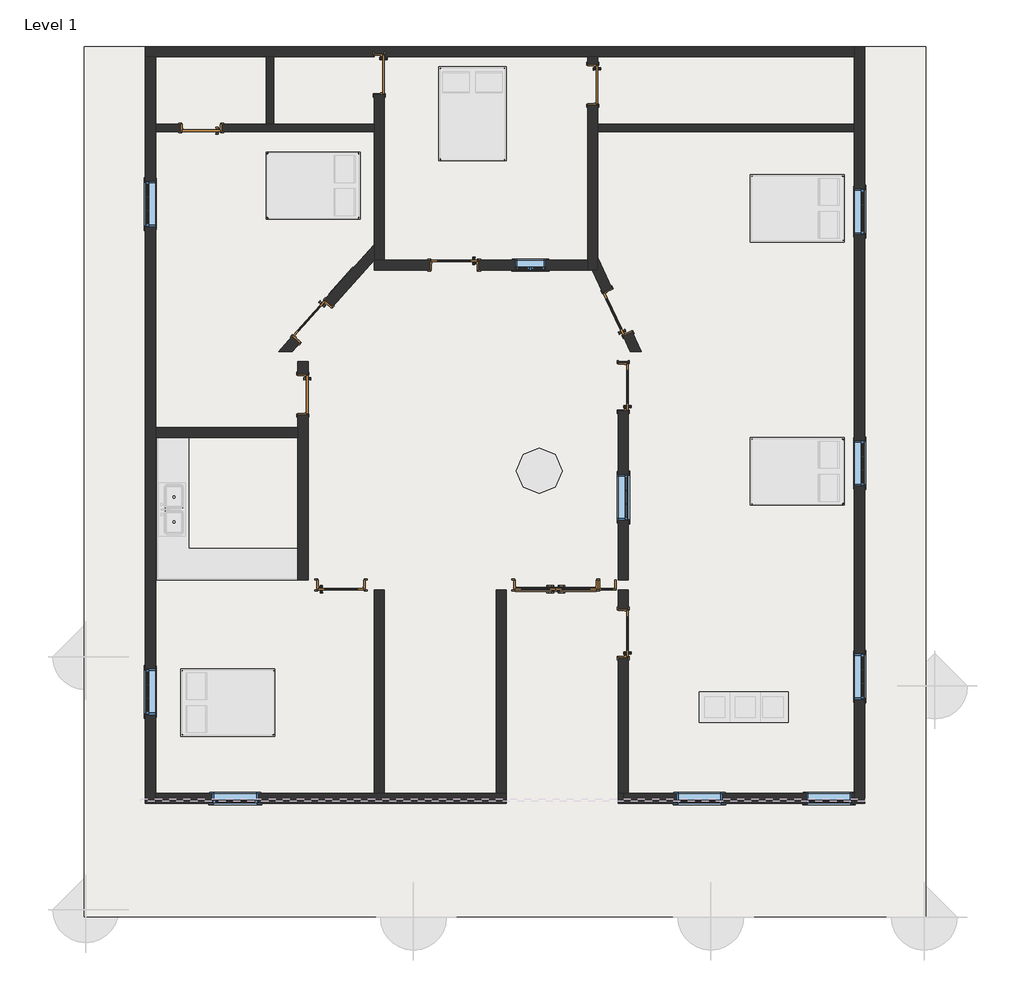
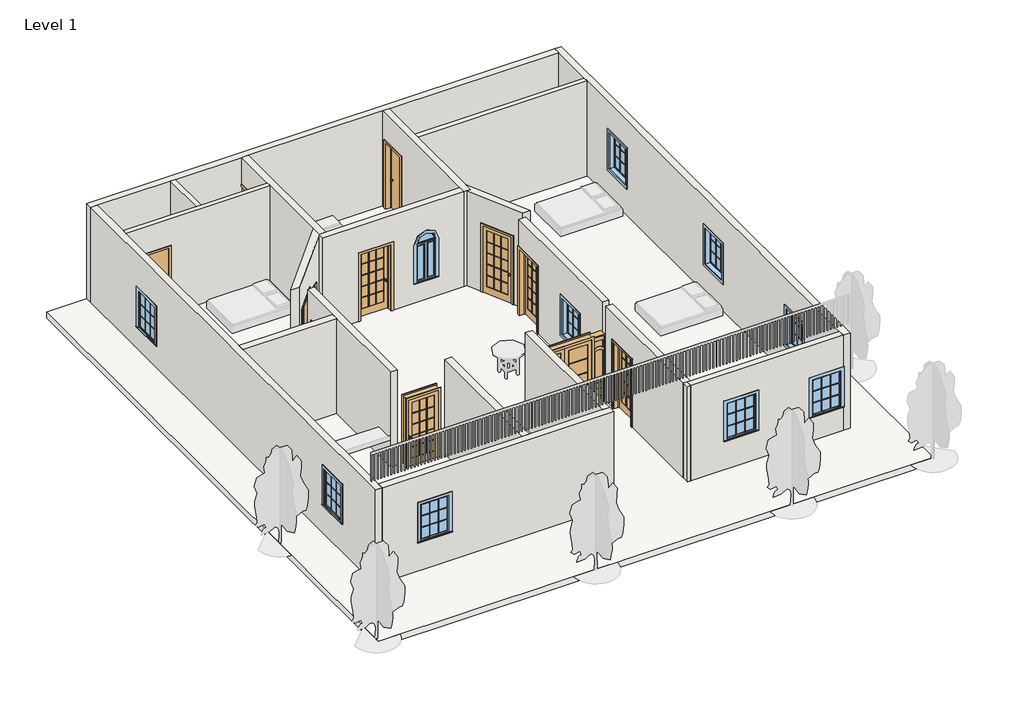
# One storey, part 1 of 3: 19 walls, 12 doors, 11 windows, 1 slab.
"""IFC4 building model written with IfcOpenShell, lengths in millimetres."""

from ifc_helpers import new_model, si_unit, frame, origin, origin_with_axes, place, context, project, spatial, polyline, circle_curve, outline, extrude, faceted_brep, transform, mapped, element, save
from ifc_brep_helpers import plane_surface, revolved_surface, advanced_brep
from components import door_c3736dc5, door_d93d7eea, door_715cd483, door_160b0797, door_6e1855c2, door_cfd81529, window_08a4fb52, window_29c06734, e_49ac7ee0

model = new_model("IFC4")

# Units and contexts
model_context = context("Model", 3, world=origin())
ifc_project = project(units=[si_unit("LENGTHUNIT", "METRE", prefix="MILLI")], contexts=[model_context])

# Site, building, storey
site = spatial("IfcSite", under=ifc_project)
building = spatial("IfcBuilding", under=site)
storey = spatial("IfcBuildingStorey", under=building, Name="Level 1", Elevation=0.0)

# Doors
placement = place(None, origin())
door_shape = door_c3736dc5(model_context)
element("IfcDoor", 1, ObjectType="12\" x 84\"", at=placement, inside=storey, context=model_context, shape_type="MappedRepresentation", body=[
    mapped(door_shape, transform((-305.2097877, 7760.2557946, 0.0), x_axis=(-1.0, 0.0, 0.0), y_axis=(0.0, -1.0, 0.0), z_axis=(0.0, 0.0, 1.0))),
])
door_2_shape = door_d93d7eea(model_context)
element("IfcDoor", 2, ObjectType="Door-Exterior-Double-Full Glass-Wood_Clad : 64\" x 84\"", at=placement, inside=storey, context=model_context, shape_type="MappedRepresentation", body=[
    mapped(door_2_shape, transform((-1333.9097877, 7760.2557946, 0.0), x_axis=(1.0, 0.0, 0.0), y_axis=(0.0, 1.0, 0.0), z_axis=(0.0, 0.0, 1.0))),
])
door_3_shape = door_715cd483(model_context)
element("IfcDoor", 3, ObjectType="Door-Interior-Single-Flush_Panel-Wood : 30\" x 84\"", at=placement, inside=storey, context=model_context, shape_type="MappedRepresentation", body=[
    mapped(door_3_shape, transform((-594.1347877, 17771.0307946, 0.0), x_axis=(0.0, -1.0, 0.0), y_axis=(1.0, 0.0, 0.0), z_axis=(0.0, 0.0, 1.0))),
])
element("IfcDoor", 4, ObjectType="Door-Interior-Single-Flush_Panel-Wood : 30\" x 84\"", at=placement, inside=storey, context=model_context, shape_type="MappedRepresentation", body=[
    mapped(door_3_shape, transform((-6385.3347877, 11573.4307946, 0.0), x_axis=(0.0, -1.0, 0.0), y_axis=(1.0, 0.0, 0.0), z_axis=(0.0, 0.0, 1.0))),
])
element("IfcDoor", 5, ObjectType="Door-Interior-Single-Flush_Panel-Wood : 30\" x 84\"", at=placement, inside=storey, context=model_context, shape_type="MappedRepresentation", body=[
    mapped(door_3_shape, transform((-4861.3347877, 17974.2307946, 0.0), x_axis=(0.0, -1.0, 0.0), y_axis=(1.0, 0.0, 0.0), z_axis=(0.0, 0.0, 1.0))),
])
door_4_shape = door_160b0797(model_context)
element("IfcDoor", 6, ObjectType="Door-Interior-Single-Flush_Panel-Wood : 30\" x 84\"", at=placement, inside=storey, context=model_context, shape_type="MappedRepresentation", body=[
    mapped(door_4_shape, transform((-8420.5097877, 16904.2557946, 0.0), x_axis=(-1.0, 0.0, 0.0), y_axis=(0.0, -1.0, 0.0), z_axis=(0.0, 0.0, 1.0))),
])
door_5_shape = door_6e1855c2(model_context)
element("IfcDoor", 7, ObjectType="Door-Interior-Single-Full Glass-Wood : 36\" x 84\"", at=placement, inside=storey, context=model_context, shape_type="MappedRepresentation", body=[
    mapped(door_5_shape, transform((-5626.5097877, 7760.2557946, 0.0), x_axis=(1.0, 0.0, 0.0), y_axis=(0.0, 1.0, 0.0), z_axis=(0.0, 0.0, 1.0))),
])
element("IfcDoor", 8, ObjectType="Door-Interior-Single-Full Glass-Wood : 36\" x 84\"", at=placement, inside=storey, context=model_context, shape_type="MappedRepresentation", body=[
    mapped(door_5_shape, transform((15.4652123, 11725.8307946, 0.0), x_axis=(0.0, 1.0, 0.0), y_axis=(-1.0, 0.0, 0.0), z_axis=(0.0, 0.0, 1.0))),
])
element("IfcDoor", 9, ObjectType="Door-Interior-Single-Full Glass-Wood : 36\" x 84\"", at=placement, inside=storey, context=model_context, shape_type="MappedRepresentation", body=[
    mapped(door_5_shape, transform((15.4652123, 6798.2307946, 0.0), x_axis=(0.0, 1.0, 0.0), y_axis=(-1.0, 0.0, 0.0), z_axis=(0.0, 0.0, 1.0))),
])
element("IfcDoor", 10, ObjectType="Door-Interior-Single-Full Glass-Wood : 36\" x 84\"", at=placement, inside=storey, context=model_context, shape_type="MappedRepresentation", body=[
    mapped(door_5_shape, transform((-3365.9097877, 14167.4057946, 0.0), x_axis=(-1.0, 0.0, 0.0), y_axis=(0.0, -1.0, 0.0), z_axis=(0.0, 0.0, 1.0))),
])
element("IfcDoor", 11, ObjectType="Door-Interior-Single-Full Glass-Wood : 36\" x 84\"", at=placement, inside=storey, context=model_context, shape_type="MappedRepresentation", body=[
    mapped(door_5_shape, transform((-6206.5889969, 13036.54514, 0.0), x_axis=(-0.666794859469825, -0.7452413135251, 0.0), y_axis=(0.7452413135251, -0.666794859469825, 0.0), z_axis=(0.0, 0.0, 1.0))),
])
door_6_shape = door_cfd81529(model_context)
element("IfcDoor", 12, ObjectType="Door-Interior-Single-Full Glass-Wood : 36\" x 84\"", at=placement, inside=storey, context=model_context, shape_type="MappedRepresentation", body=[
    mapped(door_6_shape, transform((-102.8737328, 13220.5207409, 0.0), x_axis=(-0.4226182617406977, 0.9063077870366507, 0.0), y_axis=(-0.9063077870366507, -0.4226182617406977, 0.0), z_axis=(0.0, 0.0, 1.0))),
])

# Slab
element("IfcSlab", 13, ObjectType="LW Concrete on Metal Deck", at=placement, inside=storey, context=model_context, shape_type="SweptSolid", body=[
    extrude(outline(polyline([(6057.4902123, 18533.0307946), (6057.4902123, 1134.0307946), (-10757.3097877, 1134.0307946), (-10757.3097877, 18533.0307946), (6057.4902123, 18533.0307946)])), frame((0.0, 0.0, -186.0351562), z_axis=(0.0, 0.0, 1.0), x_axis=(1.0, 0.0, 0.0)), (0.0, 0.0, 1.0), 186.0351562),
])

# Walls
element("IfcWall", 14, ObjectType="Generic - 6\"", at=placement, inside=storey, context=model_context, shape_type="Brep", body=[
    faceted_brep([(-9334.9097877, 16831.2307946, 3048.0), (-9334.9097877, 16831.2307946, 0.0), (-8826.9097877, 16831.2307946, 0.0), (-8826.9097877, 16831.2307946, 2159.0), (-8014.1097877, 16831.2307946, 2159.0), (-8014.1097877, 16831.2307946, 0.0), (-4966.1097877, 16831.2307946, 0.0), (-4966.1097877, 16831.2307946, 3048.0), (-9334.9097877, 16983.6307946, 0.0), (-9334.9097877, 16983.6307946, 3048.0), (-7125.1097877, 16983.6307946, 3048.0), (-6972.7097877, 16983.6307946, 3048.0), (-4966.1097877, 16983.6307946, 3048.0), (-4966.1097877, 16983.6307946, 0.0), (-6972.7097877, 16983.6307946, 0.0), (-7125.1097877, 16983.6307946, 0.0), (-8014.1097877, 16983.6307946, 0.0), (-8014.1097877, 16983.6307946, 2159.0), (-8826.9097877, 16983.6307946, 2159.0), (-8826.9097877, 16983.6307946, 0.0)], [[[0, 1, 2, 3, 4, 5, 6, 7]], [[8, 9, 10, 11, 12, 13, 14, 15, 16, 17, 18, 19]], [[1, 8, 19, 2]], [[13, 6, 5, 16, 15, 14]], [[1, 0, 9, 8]], [[7, 6, 13, 12]], [[18, 3, 2, 19]], [[3, 18, 17, 4]], [[4, 17, 16, 5]], [[0, 7, 12, 11, 10, 9]]]),
])
element("IfcWall", 15, ObjectType="Generic - 6\"", at=placement, inside=storey, context=model_context, shape_type="SweptSolid", body=[
    extrude(outline(polyline([(-7125.1097877, 16983.6307946), (-7125.1097877, 18329.8307946), (-6972.7097877, 18329.8307946), (-6972.7097877, 16983.6307946), (-7125.1097877, 16983.6307946)])), origin_with_axes(), (0.0, 0.0, 1.0), 3048.0),
])
element("IfcWall", 16, ObjectType="Generic - 6\"", at=placement, inside=storey, context=model_context, shape_type="SweptSolid", body=[
    extrude(outline(polyline([(4635.0902123, 16831.2307946), (-495.7097877, 16831.2307946), (-495.7097877, 16983.6307946), (4635.0902123, 16983.6307946), (4635.0902123, 16831.2307946)])), origin_with_axes(), (0.0, 0.0, 1.0), 3048.0),
])
element("IfcWall", 17, ObjectType="Generic - 8\"", at=placement, inside=storey, context=model_context, shape_type="Brep", body=[
    faceted_brep([(-9538.1097877, 18329.8307946, 3048.0), (-9538.1097877, 18329.8307946, 0.0), (-9334.9097877, 18329.8307946, 0.0), (-7125.1097877, 18329.8307946, 0.0), (-6972.7097877, 18329.8307946, 0.0), (-4966.1097877, 18329.8307946, 0.0), (-4966.1097877, 18329.8307946, 2159.0), (-4762.9097877, 18329.8307946, 2159.0), (-4762.9097877, 18329.8307946, 0.0), (-698.9097877, 18329.8307946, 0.0), (-495.7097877, 18329.8307946, 0.0), (4635.0902123, 18329.8307946, 0.0), (4635.0902123, 18329.8307946, 3048.0), (-495.7097877, 18329.8307946, 3048.0), (-698.9097877, 18329.8307946, 3048.0), (-4762.9097877, 18329.8307946, 3048.0), (-4966.1097877, 18329.8307946, 3048.0), (-6972.7097877, 18329.8307946, 3048.0), (-7125.1097877, 18329.8307946, 3048.0), (-9334.9097877, 18329.8307946, 3048.0), (4635.0902123, 18533.0307946, 0.0), (-9538.1097877, 18533.0307946, 0.0), (-9538.1097877, 18533.0307946, 3048.0), (4635.0902123, 18533.0307946, 3048.0), (-4762.9097877, 18380.6307946, 0.0), (-4966.1097877, 18380.6307946, 0.0), (-4966.1097877, 18380.6307946, 2159.0), (-4762.9097877, 18380.6307946, 2159.0)], [[[0, 1, 2, 3, 4, 5, 6, 7, 8, 9, 10, 11, 12, 13, 14, 15, 16, 17, 18, 19]], [[20, 21, 22, 23]], [[21, 20, 11, 10, 9, 8, 24, 25, 5, 4, 3, 2, 1]], [[1, 0, 22, 21]], [[12, 11, 20, 23]], [[25, 26, 6, 5]], [[27, 24, 8, 7]], [[26, 27, 7, 6]], [[26, 25, 24, 27]], [[0, 19, 18, 17, 16, 15, 14, 13, 12, 23, 22]]]),
])
element("IfcWall", 18, ObjectType="Generic - 8\"", at=placement, inside=storey, context=model_context, shape_type="Brep", body=[
    faceted_brep([(-9334.9097877, 3394.6307946, 0.0), (-9334.9097877, 3597.8307946, 0.0), (-9334.9097877, 7661.8307946, 0.0), (-9334.9097877, 7865.0307946, 0.0), (-9334.9097877, 10709.8307946, 0.0), (-9334.9097877, 10913.0307946, 0.0), (-9334.9097877, 12233.8307946, 0.0), (-9334.9097877, 12437.0307946, 0.0), (-9334.9097877, 16831.2307946, 0.0), (-9334.9097877, 16983.6307946, 0.0), (-9334.9097877, 18329.8307946, 0.0), (-9334.9097877, 18329.8307946, 3048.0), (-9334.9097877, 16983.6307946, 3048.0), (-9334.9097877, 16831.2307946, 3048.0), (-9334.9097877, 12437.0307946, 3048.0), (-9334.9097877, 12233.8307946, 3048.0), (-9334.9097877, 10913.0307946, 3048.0), (-9334.9097877, 10709.8307946, 3048.0), (-9334.9097877, 7865.0307946, 3048.0), (-9334.9097877, 7661.8307946, 3048.0), (-9334.9097877, 3597.8307946, 3048.0), (-9334.9097877, 3394.6307946, 3048.0), (-9334.9097877, 15840.6307946, 1923.320936), (-9334.9097877, 15840.6307946, 704.120936), (-9334.9097877, 14926.2307946, 704.120936), (-9334.9097877, 14926.2307946, 1923.320936), (-9334.9097877, 6087.0307946, 2133.6), (-9334.9097877, 6087.0307946, 914.4), (-9334.9097877, 5172.6307946, 914.4), (-9334.9097877, 5172.6307946, 2133.6), (-9538.1097877, 3394.6307946, 0.0), (-9538.1097877, 3394.6307946, 3048.0), (-9538.1097877, 18329.8307946, 3048.0), (-9538.1097877, 18329.8307946, 0.0), (-9538.1097877, 15840.6307946, 1923.320936), (-9538.1097877, 14926.2307946, 1923.320936), (-9538.1097877, 14926.2307946, 704.120936), (-9538.1097877, 15840.6307946, 704.120936), (-9538.1097877, 6087.0307946, 2133.6), (-9538.1097877, 5172.6307946, 2133.6), (-9538.1097877, 5172.6307946, 914.4), (-9538.1097877, 6087.0307946, 914.4)], [[[0, 1, 2, 3, 4, 5, 6, 7, 8, 9, 10, 11, 12, 13, 14, 15, 16, 17, 18, 19, 20, 21], [22, 23, 24, 25], [26, 27, 28, 29]], [[30, 31, 32, 33], [34, 35, 36, 37], [38, 39, 40, 41]], [[10, 9, 8, 7, 6, 5, 4, 3, 2, 1, 0, 30, 33]], [[11, 10, 33, 32]], [[0, 21, 31, 30]], [[23, 22, 34, 37]], [[24, 23, 37, 36]], [[25, 24, 36, 35]], [[22, 25, 35, 34]], [[27, 26, 38, 41]], [[28, 27, 41, 40]], [[29, 28, 40, 39]], [[26, 29, 39, 38]], [[21, 20, 19, 18, 17, 16, 15, 14, 13, 12, 11, 32, 31]]]),
])
element("IfcWall", 19, ObjectType="Generic - 8\"", at=placement, inside=storey, context=model_context, shape_type="Brep", body=[
    faceted_brep([(4635.0902123, 18533.0307946, 0.0), (4635.0902123, 18329.8307946, 0.0), (4635.0902123, 16983.6307946, 0.0), (4635.0902123, 16831.2307946, 0.0), (4635.0902123, 12437.0307946, 0.0), (4635.0902123, 12233.8307946, 0.0), (4635.0902123, 7865.0307946, 0.0), (4635.0902123, 7661.8307946, 0.0), (4635.0902123, 3597.8307946, 0.0), (4635.0902123, 3394.6307946, 0.0), (4635.0902123, 3394.6307946, 3048.0), (4635.0902123, 3597.8307946, 3048.0), (4635.0902123, 7661.8307946, 3048.0), (4635.0902123, 7865.0307946, 3048.0), (4635.0902123, 12233.8307946, 3048.0), (4635.0902123, 12437.0307946, 3048.0), (4635.0902123, 16831.2307946, 3048.0), (4635.0902123, 16983.6307946, 3048.0), (4635.0902123, 18329.8307946, 3048.0), (4635.0902123, 18533.0307946, 3048.0), (4635.0902123, 5477.4307946, 2133.6), (4635.0902123, 5477.4307946, 914.4), (4635.0902123, 6391.8307946, 914.4), (4635.0902123, 6391.8307946, 2133.6), (4635.0902123, 9744.6307946, 2133.6), (4635.0902123, 9744.6307946, 914.4), (4635.0902123, 10659.0307946, 914.4), (4635.0902123, 10659.0307946, 2133.6), (4635.0902123, 14773.8307946, 2133.6), (4635.0902123, 14773.8307946, 914.4), (4635.0902123, 15688.2307946, 914.4), (4635.0902123, 15688.2307946, 2133.6), (4838.2902123, 18533.0307946, 0.0), (4838.2902123, 18533.0307946, 3048.0), (4838.2902123, 3394.6307946, 3048.0), (4838.2902123, 3394.6307946, 0.0), (4838.2902123, 5477.4307946, 2133.6), (4838.2902123, 6391.8307946, 2133.6), (4838.2902123, 6391.8307946, 914.4), (4838.2902123, 5477.4307946, 914.4), (4838.2902123, 9744.6307946, 2133.6), (4838.2902123, 10659.0307946, 2133.6), (4838.2902123, 10659.0307946, 914.4), (4838.2902123, 9744.6307946, 914.4), (4838.2902123, 14773.8307946, 2133.6), (4838.2902123, 15688.2307946, 2133.6), (4838.2902123, 15688.2307946, 914.4), (4838.2902123, 14773.8307946, 914.4)], [[[0, 1, 2, 3, 4, 5, 6, 7, 8, 9, 10, 11, 12, 13, 14, 15, 16, 17, 18, 19], [20, 21, 22, 23], [24, 25, 26, 27], [28, 29, 30, 31]], [[32, 33, 34, 35], [36, 37, 38, 39], [40, 41, 42, 43], [44, 45, 46, 47]], [[9, 8, 7, 6, 5, 4, 3, 2, 1, 0, 32, 35]], [[0, 19, 33, 32]], [[10, 9, 35, 34]], [[21, 20, 36, 39]], [[22, 21, 39, 38]], [[23, 22, 38, 37]], [[20, 23, 37, 36]], [[25, 24, 40, 43]], [[26, 25, 43, 42]], [[27, 26, 42, 41]], [[24, 27, 41, 40]], [[29, 28, 44, 47]], [[30, 29, 47, 46]], [[31, 30, 46, 45]], [[28, 31, 45, 44]], [[19, 18, 17, 16, 15, 14, 13, 12, 11, 10, 34, 33]]]),
])
element("IfcWall", 20, ObjectType="Generic - 8\"", at=placement, inside=storey, context=model_context, shape_type="Brep", body=[
    faceted_brep([(-4966.1097877, 14265.8307946, 0.0), (-4966.1097877, 14265.8307946, 3048.0), (-4966.1097877, 14570.5721961, 3048.0), (-4966.1097877, 16831.2307946, 3048.0), (-4966.1097877, 16983.6307946, 3048.0), (-4966.1097877, 18329.8307946, 3048.0), (-4966.1097877, 18329.8307946, 2159.0), (-4966.1097877, 17567.8307946, 2159.0), (-4966.1097877, 17567.8307946, 0.0), (-4966.1097877, 16983.6307946, 0.0), (-4966.1097877, 16831.2307946, 0.0), (-4966.1097877, 14570.5721961, 0.0), (-4762.9097877, 14265.8307946, 3048.0), (-4762.9097877, 14265.8307946, 0.0), (-4762.9097877, 17567.8307946, 0.0), (-4762.9097877, 17567.8307946, 2159.0), (-4762.9097877, 18329.8307946, 2159.0), (-4762.9097877, 18329.8307946, 3048.0)], [[[0, 1, 2, 3, 4, 5, 6, 7, 8, 9, 10, 11]], [[12, 13, 14, 15, 16, 17]], [[13, 0, 11, 10, 9, 8, 14]], [[5, 17, 16, 6]], [[1, 0, 13, 12]], [[7, 15, 14, 8]], [[15, 7, 6, 16]], [[5, 4, 3, 2, 1, 12, 17]]]),
])
element("IfcWall", 21, ObjectType="Generic - 8\"", at=placement, inside=storey, context=model_context, shape_type="Brep", body=[
    faceted_brep([(-698.9097877, 18329.8307946, 3048.0), (-698.9097877, 18329.8307946, 0.0), (-698.9097877, 18177.4307946, 0.0), (-698.9097877, 18177.4307946, 2159.0), (-698.9097877, 17364.6307946, 2159.0), (-698.9097877, 17364.6307946, 0.0), (-698.9097877, 14265.8307946, 0.0), (-698.9097877, 14062.6307946, 0.0), (-698.9097877, 14062.6307946, 3048.0), (-698.9097877, 14265.8307946, 3048.0), (-495.7097877, 18329.8307946, 0.0), (-495.7097877, 18329.8307946, 3048.0), (-495.7097877, 16983.6307946, 3048.0), (-495.7097877, 16831.2307946, 3048.0), (-495.7097877, 14310.87915, 3048.0), (-495.7097877, 14062.6307946, 3048.0), (-495.7097877, 14062.6307946, 0.0), (-495.7097877, 14310.87915, 0.0), (-495.7097877, 16831.2307946, 0.0), (-495.7097877, 16983.6307946, 0.0), (-495.7097877, 17364.6307946, 0.0), (-495.7097877, 17364.6307946, 2159.0), (-495.7097877, 18177.4307946, 2159.0), (-495.7097877, 18177.4307946, 0.0), (-604.1560715, 14062.6307946, 0.0), (-604.1560715, 14062.6307946, 3048.0)], [[[0, 1, 2, 3, 4, 5, 6, 7, 8, 9]], [[10, 11, 12, 13, 14, 15, 16, 17, 18, 19, 20, 21, 22, 23]], [[1, 10, 23, 2]], [[16, 24, 7, 6, 5, 20, 19, 18, 17]], [[1, 0, 11, 10]], [[8, 7, 24, 16, 15, 25]], [[4, 21, 20, 5]], [[21, 4, 3, 22]], [[22, 3, 2, 23]], [[0, 9, 8, 25, 15, 14, 13, 12, 11]]]),
])
element("IfcWall", 22, ObjectType="Generic - 8\"", at=placement, inside=storey, context=model_context, shape_type="AdvancedBrep", body=[
    advanced_brep(
    [(-698.9097877, 14062.6307946, 0.0), (-698.9097877, 14062.6307946, 3048.0), (-4966.1097877, 14062.6307946, 3048.0), (-4966.1097877, 14062.6307946, 0.0), (-3848.5097877, 14062.6307946, 0.0), (-3848.5097877, 14062.6307946, 2159.0), (-2883.3097877, 14062.6307946, 2159.0), (-2883.3097877, 14062.6307946, 0.0), (-2146.7097877, 14062.6307946, 609.6), (-2146.7097877, 14062.6307946, 1847.85), (-1537.1097877, 14062.6307946, 1847.85), (-1537.1097877, 14062.6307946, 609.6), (-698.9097877, 14265.8307946, 3048.0), (-698.9097877, 14265.8307946, 0.0), (-2883.3097877, 14265.8307946, 0.0), (-2883.3097877, 14265.8307946, 2159.0), (-3848.5097877, 14265.8307946, 2159.0), (-3848.5097877, 14265.8307946, 0.0), (-4762.9097877, 14265.8307946, 0.0), (-4966.1097877, 14265.8307946, 0.0), (-4966.1097877, 14265.8307946, 3048.0), (-4762.9097877, 14265.8307946, 3048.0), (-2146.7097877, 14265.8307946, 1847.85), (-2146.7097877, 14265.8307946, 609.6), (-1537.1097877, 14265.8307946, 609.6), (-1537.1097877, 14265.8307946, 1847.85)],
    [
        (0, 1),
        (1, 2),
        (2, 3),
        (3, 4),
        (4, 5),
        (5, 6),
        (6, 7),
        (7, 0),
        (8, 9),
        (9, 10, circle_curve(frame((-1841.9097877, 14062.6307946, 1847.85), z_axis=(0.0, 1.0, 0.0), x_axis=(-1.0, 0.0, 0.0)), 304.8)),
        (10, 11),
        (11, 8),
        (12, 13),
        (13, 14),
        (14, 15),
        (15, 16),
        (16, 17),
        (17, 18),
        (18, 19),
        (19, 20),
        (20, 21),
        (21, 12),
        (22, 23),
        (23, 24),
        (24, 25),
        (25, 22, circle_curve(frame((-1841.9097877, 14265.8307946, 1847.85), z_axis=(0.0, -1.0, 0.0), x_axis=(-1.0, 0.0, 0.0)), 304.8)),
        (13, 0),
        (7, 14),
        (3, 19),
        (17, 4),
        (12, 1),
        (2, 20),
        (16, 5),
        (15, 6),
        (22, 9),
        (8, 23),
        (24, 11),
        (10, 25),
    ],
    [
        plane_surface(frame((-2578.5097877, 14062.6307946, 0.0), z_axis=(0.0, -1.0, 0.0), x_axis=(1.0, 0.0, 0.0))),
        plane_surface(frame((-2578.5097877, 14265.8307946, 0.0), z_axis=(0.0, 1.0, 0.0), x_axis=(-1.0, 0.0, 0.0))),
        plane_surface(frame((-4864.5097877, 14062.6307946, 0.0), z_axis=(0.0, 0.0, -1.0), x_axis=(0.0, 1.0, 0.0))),
        plane_surface(frame((-698.9097877, 18329.8307946, 0.0), z_axis=(1.0, 0.0, 0.0), x_axis=(0.0, -1.0, 0.0))),
        plane_surface(frame((-4966.1097877, 18329.8307946, 0.0), z_axis=(-1.0, 0.0, 0.0), x_axis=(0.0, -1.0, 0.0))),
        plane_surface(frame((-3848.5097877, 15586.6307946, 0.0), z_axis=(1.0, 0.0, 0.0), x_axis=(0.0, -1.0, 0.0))),
        plane_surface(frame((-3848.5097877, 15586.6307946, 2159.0), z_axis=(0.0, 0.0, -1.0), x_axis=(0.0, -1.0, 0.0))),
        plane_surface(frame((-2883.3097877, 15586.6307946, 2159.0), z_axis=(-1.0, 0.0, 0.0), x_axis=(0.0, -1.0, 0.0))),
        plane_surface(frame((-2146.7097877, 12741.8307946, 1847.85), z_axis=(1.0, 0.0, 0.0), x_axis=(0.0, 1.0, 0.0))),
        plane_surface(frame((-1537.1097877, 12741.8307946, 609.6), z_axis=(-1.0, 0.0, 0.0), x_axis=(0.0, 1.0, 0.0))),
        revolved_surface(polyline([(-2146.7097877, 14062.6307946, 1847.85), (-2146.7097877, 14265.8307946, 1847.85)]), (-1841.9097877, 15789.8307946, 1847.85), (0.0, -1.0, 0.0)),
        plane_surface(frame((-2146.7097877, 12741.8307946, 609.6), z_axis=(0.0, 0.0, 1.0), x_axis=(0.0, 1.0, 0.0))),
        plane_surface(frame((-9538.1097877, 18533.0307946, 3048.0), z_axis=(0.0, 0.0, 1.0), x_axis=(1.0, 0.0, 0.0))),
    ],
    [
        (0, [[1, 2, 3, 4, 5, 6, 7, 8], [9, 10, 11, 12]]),
        (1, [[13, 14, 15, 16, 17, 18, 19, 20, 21, 22], [23, 24, 25, 26]]),
        (2, [[27, -8, 28, -14]]),
        (2, [[29, -19, -18, 30, -4]]),
        (3, [[-1, -27, -13, 31]]),
        (4, [[-3, 32, -20, -29]]),
        (5, [[33, -5, -30, -17]]),
        (6, [[-33, -16, 34, -6]]),
        (7, [[-34, -15, -28, -7]]),
        (8, [[35, -9, 36, -23]]),
        (9, [[37, -11, 38, -25]]),
        (10, [[-35, -26, -38, -10]]),
        (11, [[-37, -24, -36, -12]]),
        (12, [[-2, -31, -22, -21, -32]]),
    ],
),
])
element("IfcWall", 23, ObjectType="Generic - 8\"", at=placement, inside=storey, context=model_context, shape_type="SweptSolid", body=[
    extrude(outline(polyline([(-6490.1097877, 10709.8307946), (-9334.9097877, 10709.8307946), (-9334.9097877, 10913.0307946), (-6490.1097877, 10913.0307946), (-6490.1097877, 10709.8307946)])), origin_with_axes(), (0.0, 0.0, 1.0), 3048.0),
])
element("IfcWall", 24, ObjectType="Generic - 8\"", at=placement, inside=storey, context=model_context, shape_type="Brep", body=[
    faceted_brep([(-9334.9097877, 3394.6307946, 0.0), (-2324.5097877, 3394.6307946, 0.0), (-2324.5097877, 3394.6307946, 3048.0), (-9334.9097877, 3394.6307946, 3048.0), (-8198.2597877, 3394.6307946, 2133.6), (-7283.8597877, 3394.6307946, 2133.6), (-7283.8597877, 3394.6307946, 914.4), (-8198.2597877, 3394.6307946, 914.4), (-9334.9097877, 3597.8307946, 0.0), (-9334.9097877, 3597.8307946, 3048.0), (-4966.1097877, 3597.8307946, 3048.0), (-4762.9097877, 3597.8307946, 3048.0), (-2527.7097877, 3597.8307946, 3048.0), (-2324.5097877, 3597.8307946, 3048.0), (-2324.5097877, 3597.8307946, 0.0), (-2527.7097877, 3597.8307946, 0.0), (-4762.9097877, 3597.8307946, 0.0), (-4966.1097877, 3597.8307946, 0.0), (-8198.2597877, 3597.8307946, 2133.6), (-8198.2597877, 3597.8307946, 914.4), (-7283.8597877, 3597.8307946, 914.4), (-7283.8597877, 3597.8307946, 2133.6)], [[[0, 1, 2, 3], [4, 5, 6, 7]], [[8, 9, 10, 11, 12, 13, 14, 15, 16, 17], [18, 19, 20, 21]], [[1, 0, 8, 17, 16, 15, 14]], [[0, 3, 9, 8]], [[19, 18, 4, 7]], [[20, 19, 7, 6]], [[21, 20, 6, 5]], [[18, 21, 5, 4]], [[2, 1, 14, 13]], [[3, 2, 13, 12, 11, 10, 9]]]),
])
element("IfcWall", 25, ObjectType="Generic - 8\"", at=placement, inside=storey, context=model_context, shape_type="Brep", body=[
    faceted_brep([(-6286.9097877, 12233.8307946, 0.0), (-6286.9097877, 12233.8307946, 3048.0), (-6286.9097877, 7865.0307946, 3048.0), (-6286.9097877, 7865.0307946, 0.0), (-6286.9097877, 11167.0307946, 0.0), (-6286.9097877, 11167.0307946, 2159.0), (-6286.9097877, 11979.8307946, 2159.0), (-6286.9097877, 11979.8307946, 0.0), (-6490.1097877, 12233.8307946, 3048.0), (-6490.1097877, 12233.8307946, 0.0), (-6490.1097877, 11979.8307946, 0.0), (-6490.1097877, 11979.8307946, 2159.0), (-6490.1097877, 11167.0307946, 2159.0), (-6490.1097877, 11167.0307946, 0.0), (-6490.1097877, 10913.0307946, 0.0), (-6490.1097877, 10709.8307946, 0.0), (-6490.1097877, 7865.0307946, 0.0), (-6490.1097877, 7865.0307946, 3048.0), (-6490.1097877, 10709.8307946, 3048.0), (-6490.1097877, 10913.0307946, 3048.0)], [[[0, 1, 2, 3, 4, 5, 6, 7]], [[8, 9, 10, 11, 12, 13, 14, 15, 16, 17, 18, 19]], [[9, 0, 7, 10]], [[3, 16, 15, 14, 13, 4]], [[1, 0, 9, 8]], [[3, 2, 17, 16]], [[12, 5, 4, 13]], [[5, 12, 11, 6]], [[6, 11, 10, 7]], [[2, 1, 8, 19, 18, 17]]]),
])
element("IfcWall", 26, ObjectType="Generic - 8\"", at=placement, inside=storey, context=model_context, shape_type="SweptSolid", body=[
    extrude(outline(polyline([(-4762.9097877, 7661.8307946), (-4762.9097877, 3597.8307946), (-4966.1097877, 3597.8307946), (-4966.1097877, 7661.8307946), (-4762.9097877, 7661.8307946)])), origin_with_axes(), (0.0, 0.0, 1.0), 3048.0),
])
element("IfcWall", 27, ObjectType="Generic - 8\"", at=placement, inside=storey, context=model_context, shape_type="SweptSolid", body=[
    extrude(outline(polyline([(-2527.7097877, 3597.8307946), (-2527.7097877, 7661.8307946), (-2324.5097877, 7661.8307946), (-2324.5097877, 3597.8307946), (-2527.7097877, 3597.8307946)])), origin_with_axes(), (0.0, 0.0, 1.0), 3048.0),
])
element("IfcWall", 28, ObjectType="Generic - 8\"", at=placement, inside=storey, context=model_context, shape_type="Brep", body=[
    faceted_brep([(-89.3097877, 12233.8307946, 3048.0), (-89.3097877, 12233.8307946, 0.0), (-89.3097877, 12208.4307946, 0.0), (-89.3097877, 12208.4307946, 2159.0), (-89.3097877, 11243.2307946, 2159.0), (-89.3097877, 11243.2307946, 0.0), (-89.3097877, 7865.0307946, 0.0), (-89.3097877, 7865.0307946, 3048.0), (-89.3097877, 9058.8307946, 1945.1446641), (-89.3097877, 9058.8307946, 725.9446641), (-89.3097877, 9973.2307946, 725.9446641), (-89.3097877, 9973.2307946, 1945.1446641), (113.8902123, 12233.8307946, 0.0), (113.8902123, 12233.8307946, 3048.0), (113.8902123, 7865.0307946, 3048.0), (113.8902123, 7865.0307946, 0.0), (113.8902123, 11243.2307946, 0.0), (113.8902123, 11243.2307946, 2159.0), (113.8902123, 12208.4307946, 2159.0), (113.8902123, 12208.4307946, 0.0), (113.8902123, 9058.8307946, 725.9446641), (113.8902123, 9058.8307946, 1945.1446641), (113.8902123, 9973.2307946, 1945.1446641), (113.8902123, 9973.2307946, 725.9446641)], [[[0, 1, 2, 3, 4, 5, 6, 7], [8, 9, 10, 11]], [[12, 13, 14, 15, 16, 17, 18, 19], [20, 21, 22, 23]], [[1, 12, 19, 2]], [[5, 16, 15, 6]], [[1, 0, 13, 12]], [[7, 6, 15, 14]], [[18, 3, 2, 19]], [[3, 18, 17, 4]], [[4, 17, 16, 5]], [[9, 8, 21, 20]], [[10, 9, 20, 23]], [[11, 10, 23, 22]], [[8, 11, 22, 21]], [[13, 0, 7, 14]]]),
    faceted_brep([(-89.3097877, 3597.8307946, 0.0), (-89.3097877, 3597.8307946, 3048.0), (-89.3097877, 7661.8307946, 3048.0), (-89.3097877, 7661.8307946, 0.0), (-89.3097877, 7280.8307946, 0.0), (-89.3097877, 7280.8307946, 2159.0), (-89.3097877, 6315.6307946, 2159.0), (-89.3097877, 6315.6307946, 0.0), (113.8902123, 3597.8307946, 3048.0), (113.8902123, 3597.8307946, 0.0), (113.8902123, 6315.6307946, 0.0), (113.8902123, 6315.6307946, 2159.0), (113.8902123, 7280.8307946, 2159.0), (113.8902123, 7280.8307946, 0.0), (113.8902123, 7661.8307946, 0.0), (113.8902123, 7661.8307946, 3048.0), (12.2902123, 3597.8307946, 0.0), (12.2902123, 3597.8307946, 3048.0)], [[[0, 1, 2, 3, 4, 5, 6, 7]], [[8, 9, 10, 11, 12, 13, 14, 15]], [[9, 16, 0, 7, 10]], [[13, 4, 3, 14]], [[1, 0, 16, 9, 8, 17]], [[3, 2, 15, 14]], [[5, 4, 13, 12]], [[6, 5, 12, 11]], [[7, 6, 11, 10]], [[1, 17, 8, 15, 2]]]),
])
element("IfcWall", 29, ObjectType="Generic - 8\"", at=placement, inside=storey, context=model_context, shape_type="AdvancedBrep", body=[
    advanced_brep(
    [(-6602.4045245, 12437.0307946, 3048.0), (-6602.4045245, 12437.0307946, 0.0), (-6450.3015375, 12607.0282507, 0.0), (-6450.3015375, 12607.0282507, 2159.0), (-5806.7111391, 13326.3351665, 2159.0), (-5806.7111391, 13326.3351665, 0.0), (-4966.1097877, 14265.8307946, 0.0), (-4966.1097877, 14265.8307946, 3048.0), (-5671.2184237, 13477.7682014, 1756.3724983), (-5467.9793505, 13704.9177538, 1838.0434121), (-5264.7402773, 13932.0673062, 1756.3724983), (-5264.7402773, 13932.0673062, 1228.4434121), (-5671.2184237, 13477.7682014, 1228.4434121), (-6875.0678838, 12437.0307946, 0.0), (-6875.0678838, 12437.0307946, 3048.0), (-4966.1097877, 14570.5721961, 3048.0), (-4966.1097877, 14570.5721961, 0.0), (-5958.144174, 13461.827882, 0.0), (-5958.144174, 13461.827882, 2159.0), (-6601.7345724, 12742.5209662, 2159.0), (-6601.7345724, 12742.5209662, 0.0), (-5822.6514586, 13613.2609169, 1756.3724983), (-5822.6514586, 13613.2609169, 1228.4434121), (-5416.1733122, 14067.5600216, 1228.4434121), (-5416.1733122, 14067.5600216, 1756.3724983), (-5619.4123854, 13840.4104692, 1838.0434121)],
    [
        (0, 1),
        (1, 2),
        (2, 3),
        (3, 4),
        (4, 5),
        (5, 6),
        (6, 7),
        (7, 0),
        (8, 9, circle_curve(frame((-5467.9793505, 13704.9177538, 1228.4434121), z_axis=(-0.7452413135251, 0.666794859469825, 0.0), x_axis=(-0.666794859469825, -0.7452413135251, 0.0)), 609.6)),
        (9, 10, circle_curve(frame((-5467.9793505, 13704.9177538, 1228.4434121), z_axis=(-0.7452413135251, 0.666794859469825, 0.0), x_axis=(-0.666794859469825, -0.7452413135251, 0.0)), 609.6)),
        (10, 11),
        (11, 12),
        (12, 8),
        (13, 14),
        (14, 15),
        (15, 16),
        (16, 17),
        (17, 18),
        (18, 19),
        (19, 20),
        (20, 13),
        (21, 22),
        (22, 23),
        (23, 24),
        (24, 25, circle_curve(frame((-5619.4123854, 13840.4104692, 1228.4434121), z_axis=(0.7452413135251, -0.666794859469825, 0.0), x_axis=(-0.666794859469825, -0.7452413135251, 0.0)), 609.6)),
        (25, 21, circle_curve(frame((-5619.4123854, 13840.4104692, 1228.4434121), z_axis=(0.7452413135251, -0.666794859469825, 0.0), x_axis=(-0.666794859469825, -0.7452413135251, 0.0)), 609.6)),
        (1, 13),
        (20, 2),
        (16, 6),
        (5, 17),
        (0, 14),
        (15, 7),
        (19, 3),
        (18, 4),
        (21, 8),
        (12, 22),
        (11, 23),
        (10, 24),
        (9, 25),
    ],
    [
        plane_surface(frame((-6693.3097877, 12335.4307946, 0.0), z_axis=(0.7452413135251, -0.666794859469825, 0.0), x_axis=(0.666794859469825, 0.7452413135251, 0.0))),
        plane_surface(frame((-6844.7428226, 12470.92351, 0.0), z_axis=(-0.7452413135251, 0.666794859469825, 0.0), x_axis=(-0.666794859469825, -0.7452413135251, 0.0))),
        plane_surface(frame((-6753.9249498, 12267.6844369, 0.0), z_axis=(0.0, 0.0, -1.0), x_axis=(-0.7452413135251009, 0.666794859469824, 0.0))),
        plane_surface(frame((-2578.5097877, 12437.0307946, 0.0), z_axis=(0.0, -1.0, 0.0), x_axis=(-1.0, 0.0, 0.0))),
        plane_surface(frame((-4966.1097877, 16247.0307946, -152.4), z_axis=(1.0, 0.0, 0.0), x_axis=(0.0, 1.0, 0.0))),
        plane_surface(frame((-7586.0492993, 13623.2236165, 0.0), z_axis=(0.6667948594698251, 0.7452413135250998, 0.0), x_axis=(0.7452413135250998, -0.6667948594698251, 0.0))),
        plane_surface(frame((-7586.0492993, 13623.2236165, 2159.0), z_axis=(0.0, 0.0, -1.0), x_axis=(0.7452413135250998, -0.6667948594698251, 0.0))),
        plane_surface(frame((-6942.4589009, 14342.5305324, 2159.0), z_axis=(-0.6667948594698251, -0.7452413135250998, 0.0), x_axis=(0.7452413135250998, -0.6667948594698251, 0.0))),
        plane_surface(frame((-5822.6514586, 13613.2609169, 1756.3724983), z_axis=(0.666794859469824, 0.7452413135251009, 0.0), x_axis=(0.7452413135251009, -0.666794859469824, 0.0))),
        plane_surface(frame((-5822.6514586, 13613.2609169, 1228.4434121), z_axis=(0.0, 0.0, 1.0), x_axis=(0.7452413135251009, -0.666794859469824, 0.0))),
        plane_surface(frame((-5416.1733122, 14067.5600216, 1228.4434121), z_axis=(-0.666794859469824, -0.7452413135251009, 0.0), x_axis=(0.7452413135251009, -0.666794859469824, 0.0))),
        revolved_surface(polyline([(-5874.457496851113, 13250.618649054637, 1228.4434121), (-6025.890531732805, 13386.111364475099, 1228.4434121)]), (-5619.4123854, 13840.4104692, 1228.4434121), (0.7452413135251, -0.666794859469825, 0.0)),
        revolved_surface(polyline([(-5874.457496851113, 13250.618649054637, 1228.4434121), (-6025.890531782498, 13386.11136451956, 1228.4434121)]), (-5619.4123854, 13840.4104692, 1228.4434121), (0.7452413135251, -0.666794859469825, 0.0)),
        plane_surface(frame((-9538.1097877, 18533.0307946, 3048.0), z_axis=(0.0, 0.0, 1.0), x_axis=(1.0, 0.0, 0.0))),
    ],
    [
        (0, [[1, 2, 3, 4, 5, 6, 7, 8], [9, 10, 11, 12, 13]]),
        (1, [[14, 15, 16, 17, 18, 19, 20, 21], [22, 23, 24, 25, 26]]),
        (2, [[27, -21, 28, -2]]),
        (2, [[29, -6, 30, -17]]),
        (3, [[-1, 31, -14, -27]]),
        (4, [[-7, -29, -16, 32]]),
        (5, [[33, -3, -28, -20]]),
        (6, [[-33, -19, 34, -4]]),
        (7, [[-34, -18, -30, -5]]),
        (8, [[-22, 35, -13, 36]]),
        (9, [[-23, -36, -12, 37]]),
        (10, [[-24, -37, -11, 38]]),
        (11, [[-25, -38, -10, 39]]),
        (12, [[-26, -39, -9, -35]]),
        (13, [[-8, -32, -15, -31]]),
    ],
),
])
element("IfcWall", 30, ObjectType="Generic - 8\"", at=placement, inside=storey, context=model_context, shape_type="Brep", body=[
    faceted_brep([(153.8736576, 12437.0307946, 0.0), (153.8736576, 12437.0307946, 3048.0), (-604.1560715, 14062.6307946, 3048.0), (-604.1560715, 14062.6307946, 0.0), (-396.0326499, 13616.3086765, 0.0), (-396.0326499, 13616.3086765, 2159.0), (11.8784963, 12741.5404005, 2159.0), (11.8784963, 12741.5404005, 0.0), (-495.7097877, 14310.87915, 0.0), (-495.7097877, 14310.87915, 3048.0), (378.0800507, 12437.0307946, 3048.0), (378.0800507, 12437.0307946, 0.0), (196.0402387, 12827.4164313, 0.0), (196.0402387, 12827.4164313, 2159.0), (-211.8709076, 13702.1847073, 2159.0), (-211.8709076, 13702.1847073, 0.0), (-495.7097877, 14062.6307946, 0.0), (-495.7097877, 14062.6307946, 3048.0)], [[[0, 1, 2, 3, 4, 5, 6, 7]], [[8, 9, 10, 11, 12, 13, 14, 15]], [[3, 16, 8, 15, 4]], [[11, 0, 7, 12]], [[1, 0, 11, 10]], [[3, 2, 17, 16]], [[9, 8, 16, 17]], [[14, 5, 4, 15]], [[5, 14, 13, 6]], [[6, 13, 12, 7]], [[2, 1, 10, 9, 17]]]),
])
element("IfcWall", 31, ObjectType="Generic - 8\"", at=placement, inside=storey, context=model_context, shape_type="Brep", body=[
    faceted_brep([(12.2902123, 3394.6307946, 0.0), (4635.0902123, 3394.6307946, 0.0), (4635.0902123, 3394.6307946, 3048.0), (12.2902123, 3394.6307946, 3048.0), (1079.0902123, 3394.6307946, 2133.6), (1993.4902123, 3394.6307946, 2133.6), (1993.4902123, 3394.6307946, 914.4), (1079.0902123, 3394.6307946, 914.4), (3669.8902123, 3394.6307946, 1971.5730495), (4584.2902123, 3394.6307946, 1971.5730495), (4584.2902123, 3394.6307946, 752.3730495), (3669.8902123, 3394.6307946, 752.3730495), (12.2902123, 3597.8307946, 0.0), (12.2902123, 3597.8307946, 3048.0), (113.8902123, 3597.8307946, 3048.0), (4635.0902123, 3597.8307946, 3048.0), (4635.0902123, 3597.8307946, 0.0), (113.8902123, 3597.8307946, 0.0), (1079.0902123, 3597.8307946, 2133.6), (1079.0902123, 3597.8307946, 914.4), (1993.4902123, 3597.8307946, 914.4), (1993.4902123, 3597.8307946, 2133.6), (3669.8902123, 3597.8307946, 1971.5730495), (3669.8902123, 3597.8307946, 752.3730495), (4584.2902123, 3597.8307946, 752.3730495), (4584.2902123, 3597.8307946, 1971.5730495)], [[[0, 1, 2, 3], [4, 5, 6, 7], [8, 9, 10, 11]], [[12, 13, 14, 15, 16, 17], [18, 19, 20, 21], [22, 23, 24, 25]], [[1, 0, 12, 17, 16]], [[0, 3, 13, 12]], [[2, 1, 16, 15]], [[18, 21, 5, 4]], [[21, 20, 6, 5]], [[20, 19, 7, 6]], [[19, 18, 4, 7]], [[22, 25, 9, 8]], [[25, 24, 10, 9]], [[24, 23, 11, 10]], [[23, 22, 8, 11]], [[3, 2, 15, 14, 13]]]),
])
element("IfcWall", 32, ObjectType="Generic - 8\"", at=placement, inside=storey, context=model_context, shape_type="SweptSolid", body=[
    extrude(outline(polyline([(12.2902123, 3394.6307946), (-89.3097877, 3394.6307946), (-89.3097877, 3597.8307946), (12.2902123, 3597.8307946), (12.2902123, 3394.6307946)])), origin_with_axes(), (0.0, 0.0, 1.0), 3048.0),
])

# Windows
window_shape = window_08a4fb52(model_context)
element("IfcWindow", 33, ObjectType="Archtop with Trim : 24\" x 24\"", at=placement, inside=storey, context=model_context, shape_type="MappedRepresentation", body=[
    mapped(window_shape, transform((-5535.7074668, 13781.5923245, 314.0434121), x_axis=(-0.666794859469825, -0.7452413135251, 0.0), y_axis=(0.7452413135251, -0.666794859469825, 0.0), z_axis=(0.0, 0.0, 1.0))),
])
window_2_shape = window_29c06734(model_context)
element("IfcWindow", 34, ObjectType="Casement 3x3 with Trim : 36\" x 48\"", at=placement, inside=storey, context=model_context, shape_type="MappedRepresentation", body=[
    mapped(window_2_shape, transform((-9436.5097877, 15383.4307946, -210.279064), x_axis=(0.0, 1.0, 0.0), y_axis=(-1.0, 0.0, 0.0), z_axis=(0.0, 0.0, 1.0))),
])
element("IfcWindow", 35, ObjectType="Casement 3x3 with Trim : 36\" x 48\"", at=placement, inside=storey, context=model_context, shape_type="MappedRepresentation", body=[
    mapped(window_2_shape, transform((-9436.5097877, 5629.8307946, 0.0), x_axis=(0.0, 1.0, 0.0), y_axis=(-1.0, 0.0, 0.0), z_axis=(0.0, 0.0, 1.0))),
])
element("IfcWindow", 36, ObjectType="Casement 3x3 with Trim : 36\" x 48\"", at=placement, inside=storey, context=model_context, shape_type="MappedRepresentation", body=[
    mapped(window_2_shape, transform((-7741.0597877, 3496.2307946, 0.0), x_axis=(-1.0, 0.0, 0.0), y_axis=(0.0, -1.0, 0.0), z_axis=(0.0, 0.0, 1.0))),
])
element("IfcWindow", 37, ObjectType="Casement 3x3 with Trim : 36\" x 48\"", at=placement, inside=storey, context=model_context, shape_type="MappedRepresentation", body=[
    mapped(window_2_shape, transform((1536.2902123, 3496.2307946, 0.0), x_axis=(-1.0, 0.0, 0.0), y_axis=(0.0, -1.0, 0.0), z_axis=(0.0, 0.0, 1.0))),
])
element("IfcWindow", 38, ObjectType="Casement 3x3 with Trim : 36\" x 48\"", at=placement, inside=storey, context=model_context, shape_type="MappedRepresentation", body=[
    mapped(window_2_shape, transform((4127.0902123, 3496.2307946, -162.0269505), x_axis=(-1.0, 0.0, 0.0), y_axis=(0.0, -1.0, 0.0), z_axis=(0.0, 0.0, 1.0))),
])
element("IfcWindow", 39, ObjectType="Casement 3x3 with Trim : 36\" x 48\"", at=placement, inside=storey, context=model_context, shape_type="MappedRepresentation", body=[
    mapped(window_2_shape, transform((4736.6902123, 5934.6307946, 0.0), x_axis=(0.0, -1.0, 0.0), y_axis=(1.0, 0.0, 0.0), z_axis=(0.0, 0.0, 1.0))),
])
element("IfcWindow", 40, ObjectType="Casement 3x3 with Trim : 36\" x 48\"", at=placement, inside=storey, context=model_context, shape_type="MappedRepresentation", body=[
    mapped(window_2_shape, transform((4736.6902123, 10201.8307946, 0.0), x_axis=(0.0, -1.0, 0.0), y_axis=(1.0, 0.0, 0.0), z_axis=(0.0, 0.0, 1.0))),
])
element("IfcWindow", 41, ObjectType="Casement 3x3 with Trim : 36\" x 48\"", at=placement, inside=storey, context=model_context, shape_type="MappedRepresentation", body=[
    mapped(window_2_shape, transform((4736.6902123, 15231.0307946, 0.0), x_axis=(0.0, -1.0, 0.0), y_axis=(1.0, 0.0, 0.0), z_axis=(0.0, 0.0, 1.0))),
])
element("IfcWindow", 42, ObjectType="Casement 3x3 with Trim : 36\" x 48\"", at=placement, inside=storey, context=model_context, shape_type="MappedRepresentation", body=[
    mapped(window_2_shape, transform((12.2902123, 9516.0307946, -188.4553359), x_axis=(0.0, -1.0, 0.0), y_axis=(1.0, 0.0, 0.0), z_axis=(0.0, 0.0, 1.0))),
])
e_shape = e_49ac7ee0(model_context)
element("IfcWindow", 43, ObjectType="e", at=placement, inside=storey, context=model_context, shape_type="MappedRepresentation", body=[
    mapped(e_shape, transform((-1833.9076296, 14164.2307946, 304.8), x_axis=(-1.0, 0.0, 0.0), y_axis=(0.0, -1.0, 0.0), z_axis=(0.0, 0.0, 1.0))),
])

save(model, "model.ifc")

# Revit data of these elements
# Type "12\" x 84\""
#   Type Mark = "10"
#   Assembly Code = "B2030100"
#   Analytic Construction = "French door, wood frame with single glass"
#   Radius = 0' - 6 89/256"
#   Lock Rail = 0' - 7 1/8"
#   Thickness = 0' - 1 3/8"
#   Thermal Resistance (R) = 1.0696 (h·ft²·°F)/BTU
#   Stiles = 0' - 1 3/8"
#   Rough Width = 1' - 2"
#   Rough Height = 7' - 1"
#   Height = 7' - 0"
#   Width = 1' - 0"
#   Heat Transfer Coefficient (U) = 0.9350 BTU/(h·ft²·°F)
#   Door Offset [instance default] = 0' - 0"
#   Bottom Rail = 0' - 9 1/2"
#   Function = 1
#   Trim Material = Cherry
#   Panel Material = Cherry
#   Glazing = Glass
#   Frame Material = Cherry
#   Visual Light Transmittance = 0
#   Solar Heat Gain Coefficient = 0
#   Wall Closure = (empty or 0)
#   Construction Type = (empty or 0)
# Type "Door-Exterior-Double-Full Glass-Wood_Clad : 64\" x 84\""
#   Type Mark = "9"
#   Assembly Code = "B2030100"
#   Analytic Construction = "French door, wood frame with double glass"
#   Top Rail = 0' - 4 11/16"
#   Threshold Offset [instance default] = 0' - 0 1/2"
#   Thickness = 0' - 1 3/8"
#   Thermal Resistance (R) = 1.9158 (h·ft²·°F)/BTU
#   Swing Angle [instance default] = 90.00°
#   Stiles = 0' - 4 3/4"
#   Rough Width = 5' - 6"
#   Rough Height = 7' - 1"
#   Panel Width = 2' - 8"
#   Door Offset [instance default] = 0' - 0"
#   Height = 7' - 0"
#   Width = 5' - 4"
#   Heat Transfer Coefficient (U) = 0.5220 BTU/(h·ft²·°F)
#   Bottom Rail = 0' - 9 1/8"
#   Exterior Trim [instance default] = yes
#   Threshold [instance default] = yes
#   Show Grill [instance default] = yes
#   Function = 1
#   Trim Material = Cherry
#   Threshold Material = Cherry
#   Panel Material = Cherry
#   Glazing = Glass
#   Frame Material = Cherry
#   Door Handle Material = Aluminum
#   Visual Light Transmittance = 0
#   Solar Heat Gain Coefficient = 0
#   Wall Closure = (empty or 0)
#   Construction Type = (empty or 0)
# Type "Door-Interior-Single-Flush_Panel-Wood : 30\" x 84\""
#   Type Mark = "12"
#   Assembly Code = "C1020300"
#   Analytic Construction = "Wooden"
#   Thickness = 0' - 1 3/8"
#   Thermal Resistance (R) = 2.5876 (h·ft²·°F)/BTU
#   Swing Angle [instance default] = 90.00°
#   Rough Width = 2' - 8"
#   Rough Height = 7' - 1"
#   Height = 7' - 0"
#   Width = 2' - 6"
#   Heat Transfer Coefficient (U) = 0.3865 BTU/(h·ft²·°F)
#   Trim Material = Cherry
#   Panel Material = Cherry
#   Frame Material = Cherry
#   Door Handle Material = Aluminum
#   Visual Light Transmittance = 0
#   Solar Heat Gain Coefficient = 0
#   Wall Closure = (empty or 0)
#   Function = (empty or 0)
# Type "Door-Interior-Single-Full Glass-Wood : 36\" x 84\""
#   Type Mark = "11"
#   Assembly Code = "C1020300"
#   Analytic Construction = "Wood frame with single clear glass"
#   Top Rail = 0' - 4 11/16"
#   Thickness = 0' - 1 3/8"
#   Thermal Resistance (R) = 1.0102 (h·ft²·°F)/BTU
#   Swing Angle [instance default] = 90.00°
#   Stiles = 0' - 4 3/4"
#   Rough Width = 3' - 2"
#   Rough Height = 7' - 1"
#   Height = 7' - 0"
#   Width = 3' - 0"
#   Heat Transfer Coefficient (U) = 0.9900 BTU/(h·ft²·°F)
#   Bottom Rail = 0' - 9 1/8"
#   Show Grill [instance default] = yes
#   Trim Material = Cherry
#   Panel Material = Cherry
#   Frame Material = Cherry
#   Door Handle Material = Aluminum
#   Visual Light Transmittance = 0
#   Solar Heat Gain Coefficient = 0
#   Wall Closure = (empty or 0)
#   Function = (empty or 0)
# Type "LW Concrete on Metal Deck"
#   Assembly Code = "B1010"
#   Function = 0
#   Layers, outside or top first: 0' - 7 51/256" "Concrete, Lightweight" (function 1); 0' - 0 1/8" "Metal Deck" (function 1)
# Type "Generic - 6\""
#   Assembly Code = "B2010"
#   Layers, outside or top first: 0' - 6" no material (function 1)
# Type "Generic - 8\""
#   Assembly Code = "B2010"
#   Layers, outside or top first: 0' - 8" no material (function 1)
# Type "Archtop with Trim : 24\" x 24\""
#   Type Mark = "15"
#   Construction Type Id = "GSP4R"
#   Assembly Code = "B2020100"
#   Analytic Construction = "1/8 in Pilkington single glazing"
#   Visual Light Transmittance = 0.9
#   Solar Heat Gain Coefficient = 0.78
#   Heat Transfer Coefficient (U) = 0.6496 BTU/(h·ft²·°F)
#   Height = 2' - 0"
#   Radius = 2' - 0"
#   Default Sill Height = 3' - 0"
#   Trim Projection - Ext. = 0' - 0 1/2"
#   Trim Projection - Int. = 0' - 0 3/4"
#   Trim Width - Exterior = 0' - 3 1/2"
#   Trim Width - Interior = 0' - 3 1/2"
#   Width = 2' - 0"
#   Define Thermal Properties by = 1
#   Glass Pane Material = Glass
#   Sash Material = Sash
#   Trim Exterior Material = Trim
#   Trim Interior Material = Trim
#   Wall Closure = (empty or 0)
# Type "Casement 3x3 with Trim : 36\" x 48\""
#   Type Mark = "21"
#   Construction Type Id = "GSP4R"
#   Assembly Code = "B2020100"
#   Analytic Construction = "1/8 in Pilkington single glazing"
#   Visual Light Transmittance = 0.9
#   Solar Heat Gain Coefficient = 0.78
#   Heat Transfer Coefficient (U) = 0.6496 BTU/(h·ft²·°F)
#   Height = 4' - 0"
#   Default Sill Height = 3' - 0"
#   Trim Projection - Ext. = 0' - 0 1/2"
#   Trim Projection - Int. = 0' - 0 3/4"
#   Trim Width - Exterior = 0' - 3 1/2"
#   Trim Width - Interior = 0' - 3 1/2"
#   Width = 3' - 0"
#   Window Inset = 0' - 0 3/4"
#   Define Thermal Properties by = 1
#   Glass Pane Material = Glass
#   Sash Material = Sash
#   Trim Exterior Material = Trim
#   Trim Interior Material = Trim
#   Wall Closure = (empty or 0)
# Type "e"
#   Type Mark = "14"
#   Construction Type Id = "SGL"
#   Assembly Code = "B2020100"
#   Analytic Construction = "Large single-glazed windows"
#   Visual Light Transmittance = 0.9
#   Solar Heat Gain Coefficient = 0.86
#   Heat Transfer Coefficient (U) = 0.979472 BTU/(h·ft²·°F)
#   Height = 4' - 0"
#   Default Sill Height = 1' - 0"
#   Trim Projection - Ext. = 0' - 0 1/2"
#   Trim Projection - Int. = 0' - 0 3/4"
#   Trim Width - Exterior = 0' - 3 1/2"
#   Trim Width - Interior = 0' - 3 1/2"
#   Width = 2' - 0"
#   Window Inset = 0' - 0 3/4"
#   Define Thermal Properties by = 1
#   Glass Pane Material = Glass
#   Sash Material = Sash
#   Trim Exterior Material = Trim
#   Trim Interior Material = Trim
#   Wall Closure = (empty or 0)
# Element 1 (IfcDoor, "12\" x 84\"")
#   Door Offset = 0' - 0"
#   Phase Created = New Construction
#   Materials on its faces: "Cherry", "Glass"
# Element 2 (IfcDoor, "Door-Exterior-Double-Full Glass-Wood_Clad : 64\" x 84\"")
#   Threshold Offset = 0' - 0 1/2"
#   Swing Angle = 90.00°
#   Door Offset = 0' - 0"
#   Threshold = yes
#   Show Grill = yes
#   Exterior Trim = yes
#   Phase Created = New Construction
#   Materials on its faces: "Cherry", "Aluminum", "Glass"
# Elements 3, 4, 5, 6 (IfcDoor, "Door-Interior-Single-Flush_Panel-Wood : 30\" x 84\"")
#   Swing Angle = 90.00°
#   Phase Created = New Construction
#   Materials on its faces: "Cherry", "Aluminum"
# Elements 7, 8, 9, 10, 11, 12 (IfcDoor, "Door-Interior-Single-Full Glass-Wood : 36\" x 84\"")
#   Swing Angle = 90.00°
#   Show Grill = yes
#   Phase Created = New Construction
#   Materials on its faces: "Cherry", "Aluminum", "Glass"
# Element 13 (IfcSlab, "LW Concrete on Metal Deck")
#   Height Offset From Level = 0' - 0"
#   Phase Created = New Construction
#   Materials on its faces: "Metal Deck", "Concrete, Lightweight"
# Elements 14, 15, 16 (IfcWall, "Generic - 6\"")
#   Top Offset = 0' - 0"
#   Base Offset = 0' - 0"
#   Unconnected Height = 10' - 0"
#   wall height = 10' - 0"
#   Phase Created = New Construction
#   Base Constraint = Level 1
#   Materials on its faces: "Default Wall", "Carpet (1)"
# Elements 17, 18, 19 (IfcWall, "Generic - 8\"")
#   Top Offset = 0' - 0"
#   Base Offset = 0' - 0"
#   Unconnected Height = 10' - 0"
#   wall height = 10' - 0"
#   Phase Created = New Construction
#   Base Constraint = Level 1
#   Materials on its faces: "Default Wall", "Plywood, Sheathing", "Carpet (1)"
# Elements 20, 21, 22, 23, 25, 26, 27, 29, 30, 32 (IfcWall, "Generic - 8\"")
#   Top Offset = 0' - 0"
#   Base Offset = 0' - 0"
#   Unconnected Height = 10' - 0"
#   wall height = 10' - 0"
#   Phase Created = New Construction
#   Base Constraint = Level 1
#   Materials on its faces: "Default Wall", "Carpet (1)"
# Elements 24, 31 (IfcWall, "Generic - 8\"")
#   Top Offset = 0' - 0"
#   Base Offset = 0' - 0"
#   Unconnected Height = 10' - 0"
#   wall height = 10' - 0"
#   Phase Created = New Construction
#   Base Constraint = Level 1
#   Materials on its faces: "Default Wall", "Carpet (1)", "Plywood, Sheathing"
# Element 28 (IfcWall, "Generic - 8\"")
#   Top Offset = 0' - 0"
#   Base Offset = 0' - 0"
#   Unconnected Height = 10' - 0"
#   wall height = 10' - 0"
#   Phase Created = New Construction
#   Base Constraint = Level 1
#   Materials on its faces: "Default Wall", "Sash", "Carpet (1)"
# Element 33 (IfcWindow, "Archtop with Trim : 24\" x 24\"")
#   Mark = "4"
#   Phase Created = New Construction
#   Materials on its faces: "Sash", "Trim", "Glass"
# Element 34 (IfcWindow, "Casement 3x3 with Trim : 36\" x 48\"")
#   Mark = "5"
#   Phase Created = New Construction
#   Materials on its faces: "Sash", "Glass", "Trim"
# Element 35 (IfcWindow, "Casement 3x3 with Trim : 36\" x 48\"")
#   Mark = "6"
#   Phase Created = New Construction
#   Materials on its faces: "Sash", "Glass", "Trim"
# Element 36 (IfcWindow, "Casement 3x3 with Trim : 36\" x 48\"")
#   Mark = "7"
#   Phase Created = New Construction
#   Materials on its faces: "Sash", "Glass", "Trim"
# Element 37 (IfcWindow, "Casement 3x3 with Trim : 36\" x 48\"")
#   Mark = "8"
#   Phase Created = New Construction
#   Materials on its faces: "Sash", "Glass", "Trim"
# Element 38 (IfcWindow, "Casement 3x3 with Trim : 36\" x 48\"")
#   Mark = "9"
#   Phase Created = New Construction
#   Materials on its faces: "Sash", "Glass", "Trim"
# Element 39 (IfcWindow, "Casement 3x3 with Trim : 36\" x 48\"")
#   Mark = "10"
#   Phase Created = New Construction
#   Materials on its faces: "Sash", "Glass", "Trim"
# Element 40 (IfcWindow, "Casement 3x3 with Trim : 36\" x 48\"")
#   Mark = "11"
#   Phase Created = New Construction
#   Materials on its faces: "Sash", "Glass", "Trim"
# Element 41 (IfcWindow, "Casement 3x3 with Trim : 36\" x 48\"")
#   Mark = "12"
#   Phase Created = New Construction
#   Materials on its faces: "Sash", "Glass", "Trim"
# Element 42 (IfcWindow, "Casement 3x3 with Trim : 36\" x 48\"")
#   Mark = "13"
#   Phase Created = New Construction
#   Materials on its faces: "Sash", "Glass", "Trim"
# Element 43 (IfcWindow, "e")
#   Mark = "1"
#   Phase Created = New Construction
#   Materials on its faces: "Sash", "Trim", "Glass"
# Materials
#   "Cherry": class "Wood", colour RGB 226 177 128, transparency 0, Description = "Prunus Serotina", Cost = 0
#   "Glass": class "Glass", colour RGB 0 128 192, transparency 0.75, Description = "Soda Lime Glass", Cost = 0
#   "Aluminum": class "Metal", colour RGB 247 247 247, transparency 0, Description = "Aluminum 6061", Cost = 0
#   "Concrete, Lightweight": class "Concrete", colour RGB 142 141 140, transparency 0, Description = "Lightweight concrete", Cost = 0
#   "Metal Deck": class "Metal", colour RGB 199 199 199, transparency 0, Description = "Steel, mill finish", Cost = 0
#   "Sash": class "Wood", colour RGB 224 178 126, transparency 0
#   "Trim": class "Wood", colour RGB 224 178 126, transparency 0
#   "Default Wall": colour RGB 128 128 128, transparency 0
#   "Carpet (1)": class "Carpet", colour RGB 124 80 67, transparency 0, Description = "Interior finish"
#   "Plywood, Sheathing": class "Wood", colour RGB 212 179 113, transparency 0, Description = "Plywood, sheathing grade", Cost = 0
